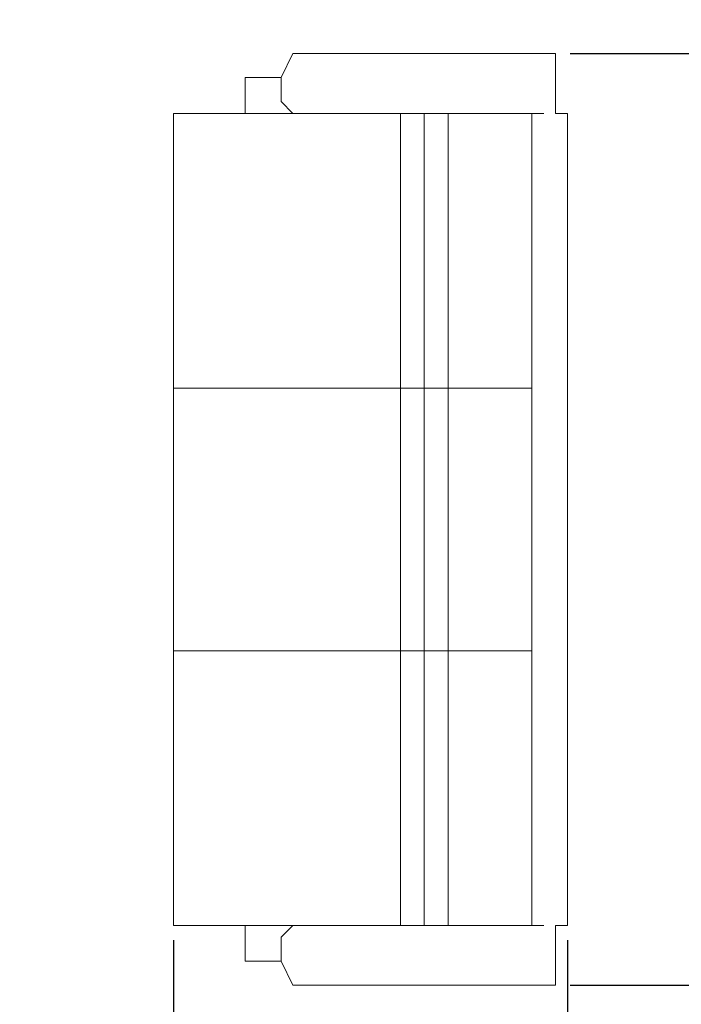
# Model space of a CAD drawing. Units: inches. Extents: x 2923 to 3500, y 1684 to 2381.
# Tile 6 of 12: x 3218 to 3246, y 1888 to 1930. Entities that reach past the tile are written whole.
import ezdxf

# ---------------------------------------------------------------- set-up
doc = ezdxf.new("R2010")
doc.units = ezdxf.units.IN
doc.layers.add('A-ANNO-DIMS', color=2, linetype='Continuous', lineweight=18)
doc.layers.add('Furniture', color=7, linetype='Continuous', lineweight=15)
doc.styles.get("Standard").update_dxf_attribs({"font": 'txt', "height": 5})
doc.dimstyles.new('ISO-25', dxfattribs={"dimtxt": 5, "dimasz": 2.5, "dimexe": 1.25, "dimexo": 0.625, "dimtad": 1, "dimlunit": 3, "dimtxsty": 'Standard', "dimcen": 2.5, "dimadec": 0, "dimazin": 0, "dimtfac": 1, "dimtmove": 0, "dimatfit": 3, "dimfxl": 1, "dimarcsym": 0})

# ---------------------------------------------------------------- blocks, each defined once
blk = doc.blocks.new('*D45')
at = {"layer": 'A-ANNO-DIMS', "color": 0, "lineweight": -2, "transparency": 16777216}
for p, q in [((3227.902, 1933.562), (3227.902, 1931.16)), ((3239.752, 1933.562), (3239.752, 1931.16)), ((3230.402, 1932.41), (3237.252, 1932.41)), ((3239.752, 1932.41), (3310.644, 1932.41))]:
    blk.add_line(p, q, dxfattribs=at)
at = {"layer": 'A-ANNO-DIMS', "color": 0, "transparency": 16777216}
for points in [[(3230.402, 1932.827), (3230.402, 1931.993), (3227.902, 1932.41)], [(3237.252, 1932.827), (3237.252, 1931.993), (3239.752, 1932.41)]]:
    blk.add_solid(points, dxfattribs=at)
at = {"layer": 'Defpoints', "color": 0, "transparency": 16777216}
for p in [(3227.902, 1934.187), (3239.752, 1934.187), (3239.752, 1932.41)]:
    blk.add_point(p, dxfattribs=at)
at = {"layer": 'A-ANNO-DIMS', "color": 0, "transparency": 16777216, "insert": (3276.448, 1936.011), "char_height": 5, "attachment_point": 5}
blk.add_mtext('TABLE 1\'-0" TYP.', dxfattribs=at)
blk = doc.blocks.new('*D54')
at = {"layer": 'A-ANNO-DIMS', "color": 0, "lineweight": -2, "transparency": 16777216}
for p, q in [((3166.316, 2236.755), (3166.316, 1685.656)), ((3193.644, 2236.755), (3193.644, 1685.656)), ((3168.816, 1686.906), (3191.144, 1686.906)), ((3193.644, 1686.906), (3235.489, 1686.906))]:
    blk.add_line(p, q, dxfattribs=at)
at = {"layer": 'A-ANNO-DIMS', "color": 0, "transparency": 16777216}
for points in [[(3168.816, 1687.323), (3168.816, 1686.49), (3166.316, 1686.906)], [(3191.144, 1687.323), (3191.144, 1686.49), (3193.644, 1686.906)]]:
    blk.add_solid(points, dxfattribs=at)
at = {"layer": 'Defpoints', "color": 0, "transparency": 16777216}
for p in [(3166.316, 2237.38), (3193.644, 2237.38), (3193.644, 1686.906)]:
    blk.add_point(p, dxfattribs=at)
at = {"layer": 'A-ANNO-DIMS', "color": 0, "transparency": 16777216, "insert": (3215.817, 1691.341), "char_height": 5, "attachment_point": 5}
blk.add_mtext('2\'-3 1/2"', dxfattribs=at)
blk = doc.blocks.new('*D60')
at = {"layer": 'A-ANNO-DIMS', "color": 0, "lineweight": -2, "transparency": 16777216}
for p, q in [((3241.344, 1928.122), (3479.98, 1928.122)), ((3478.73, 1925.622), (3478.73, 1891.08)), ((3241.344, 1888.58), (3479.98, 1888.58))]:
    blk.add_line(p, q, dxfattribs=at)
at = {"layer": 'A-ANNO-DIMS', "color": 0, "transparency": 16777216}
for points in [[(3478.313, 1925.622), (3479.146, 1925.622), (3478.73, 1928.122)], [(3478.313, 1891.08), (3479.146, 1891.08), (3478.73, 1888.58)]]:
    blk.add_solid(points, dxfattribs=at)
at = {"layer": 'Defpoints', "color": 0, "transparency": 16777216}
for p in [(3240.719, 1928.122), (3240.719, 1888.58), (3478.73, 1888.58)]:
    blk.add_point(p, dxfattribs=at)
at = {"layer": 'A-ANNO-DIMS', "color": 0, "transparency": 16777216, "insert": (3474.295, 1908.351), "char_height": 5, "attachment_point": 5, "rotation": 90}
blk.add_mtext('3\'-3 1/2"', dxfattribs=at)
blk = doc.blocks.new('*D61')
at = {"layer": 'A-ANNO-DIMS', "color": 0, "lineweight": -2, "transparency": 16777216}
for p, q in [((3224.497, 1890.49), (3224.497, 1685.656)), ((3241.226, 1890.49), (3241.226, 1685.656)), ((3226.997, 1686.906), (3238.726, 1686.906)), ((3241.226, 1686.906), (3282.119, 1686.906))]:
    blk.add_line(p, q, dxfattribs=at)
at = {"layer": 'A-ANNO-DIMS', "color": 0, "transparency": 16777216}
for points in [[(3226.997, 1687.323), (3226.997, 1686.49), (3224.497, 1686.906)], [(3238.726, 1687.323), (3238.726, 1686.49), (3241.226, 1686.906)]]:
    blk.add_solid(points, dxfattribs=at)
at = {"layer": 'Defpoints', "color": 0, "transparency": 16777216}
for p in [(3224.497, 1891.115), (3241.226, 1891.115), (3241.226, 1686.906)]:
    blk.add_point(p, dxfattribs=at)
at = {"layer": 'A-ANNO-DIMS', "color": 0, "transparency": 16777216, "insert": (3262.923, 1691.341), "char_height": 5, "attachment_point": 5}
blk.add_mtext('1\'-4 1/2"', dxfattribs=at)
blk = doc.blocks.new('*D62')
at = {"layer": 'A-ANNO-DIMS', "color": 0, "lineweight": -2, "transparency": 16777216}
for p, q in [((3204.334, 1920.391), (3204.334, 2370.156)), ((3217.261, 1920.391), (3217.261, 2370.156)), ((3206.834, 2368.906), (3214.761, 2368.906)), ((3217.261, 2368.906), (3238.868, 2368.906))]:
    blk.add_line(p, q, dxfattribs=at)
at = {"layer": 'A-ANNO-DIMS', "color": 0, "transparency": 16777216}
for points in [[(3206.834, 2369.323), (3206.834, 2368.49), (3204.334, 2368.906)], [(3214.761, 2369.323), (3214.761, 2368.49), (3217.261, 2368.906)]]:
    blk.add_solid(points, dxfattribs=at)
at = {"layer": 'Defpoints', "color": 0, "transparency": 16777216}
for p in [(3217.261, 2368.906), (3204.334, 1919.766), (3217.261, 1919.766)]:
    blk.add_point(p, dxfattribs=at)
at = {"layer": 'A-ANNO-DIMS', "color": 0, "transparency": 16777216, "insert": (3229.315, 2372.507), "char_height": 5, "attachment_point": 5}
blk.add_mtext('1\'-1"', dxfattribs=at)

msp = doc.modelspace()

# ---------------------------------------------------------------- linework, layer by layer
at = {"layer": 'Furniture'}
for p, q in [((3229.06, 1927.108), (3229.567, 1928.122)), ((3229.567, 1928.122), (3240.719, 1928.122)), ((3240.719, 1928.122), (3240.719, 1925.587)), ((3227.539, 1925.587), (3227.539, 1927.108)), ((3227.539, 1927.108), (3229.06, 1927.108)), ((3229.06, 1927.108), (3229.06, 1926.094)), ((3229.06, 1926.094), (3229.567, 1925.587)), ((3224.497, 1891.115), (3224.497, 1925.587)), ((3224.497, 1925.587), (3227.539, 1925.587)), ((3227.539, 1925.587), (3229.567, 1925.587)), ((3229.567, 1925.587), (3240.212, 1925.587)), ((3234.129, 1891.115), (3234.129, 1925.587)), ((3235.143, 1891.115), (3235.143, 1925.587)), ((3236.157, 1891.115), (3236.157, 1925.587)), ((3239.706, 1925.587), (3239.706, 1891.115)), ((3240.719, 1925.587), (3241.226, 1925.587)), ((3241.226, 1925.587), (3241.226, 1891.115)), ((3224.497, 1913.927), (3239.706, 1913.927)), ((3224.497, 1902.775), (3239.706, 1902.775)), ((3227.539, 1891.115), (3224.497, 1891.115)), ((3227.539, 1891.115), (3229.567, 1891.115)), ((3227.539, 1889.594), (3227.539, 1891.115)), ((3229.06, 1890.608), (3229.567, 1891.115)), ((3229.567, 1891.115), (3240.212, 1891.115)), ((3241.226, 1891.115), (3240.719, 1891.115)), ((3240.719, 1891.115), (3240.719, 1888.58)), ((3229.06, 1889.594), (3229.06, 1890.608)), ((3229.06, 1889.594), (3227.539, 1889.594)), ((3229.567, 1888.58), (3229.06, 1889.594)), ((3240.719, 1888.58), (3229.567, 1888.58))]:
    msp.add_line(p, q, dxfattribs=at)

# ---------------------------------------------------------------- dimensions: what is measured, and where the dimension line sits
at = {"layer": 'A-ANNO-DIMS'}
for base, p1, p2, picture, middle in [((3217.261, 2368.906), (3204.334, 1919.766), (3217.261, 1919.766), '*D62', (3229.315, 2372.507)), ((3193.644, 1686.906), (3166.316, 2237.38), (3193.644, 2237.38), '*D54', (3215.817, 1691.341)), ((3241.226, 1686.906), (3224.497, 1891.115), (3241.226, 1891.115), '*D61', (3262.923, 1691.341))]:
    dim = msp.add_linear_dim(base=base, p1=p1, p2=p2, dimstyle='ISO-25', override={"dimdec": 1, "dimlfac": 1, "dimrnd": 0, "dimzin": 1, "dimdsep": 46, "dimlunit": 4, "dimfrac": 2}, dxfattribs=at)
    dim.commit()
    dim.dimension.update_dxf_attribs({"geometry": picture, "text_midpoint": middle})
dim = msp.add_linear_dim(base=(3239.7515, 1932.41), p1=(3227.9018, 1934.1875), p2=(3239.7515, 1934.1875), text='TABLE <> TYP.', dimstyle='ISO-25', override={"dimdec": 1, "dimlfac": 1, "dimrnd": 0, "dimzin": 1, "dimdsep": 46, "dimlunit": 4, "dimfrac": 2}, dxfattribs=at)
dim.commit()
dim.dimension.update_dxf_attribs({"geometry": '*D45', "text_midpoint": (3276.4479, 1936.0112)})
dim = msp.add_linear_dim(base=(3478.73, 1888.58), p1=(3240.719, 1928.122), p2=(3240.719, 1888.58), angle=90, dimstyle='ISO-25', override={"dimdec": 1, "dimlfac": 1, "dimrnd": 0, "dimzin": 1, "dimdsep": 46, "dimlunit": 4, "dimfrac": 2}, dxfattribs=at)
dim.commit()
dim.dimension.update_dxf_attribs({"geometry": '*D60', "text_midpoint": (3474.295, 1908.351)})

doc.saveas('drawing.dxf')
